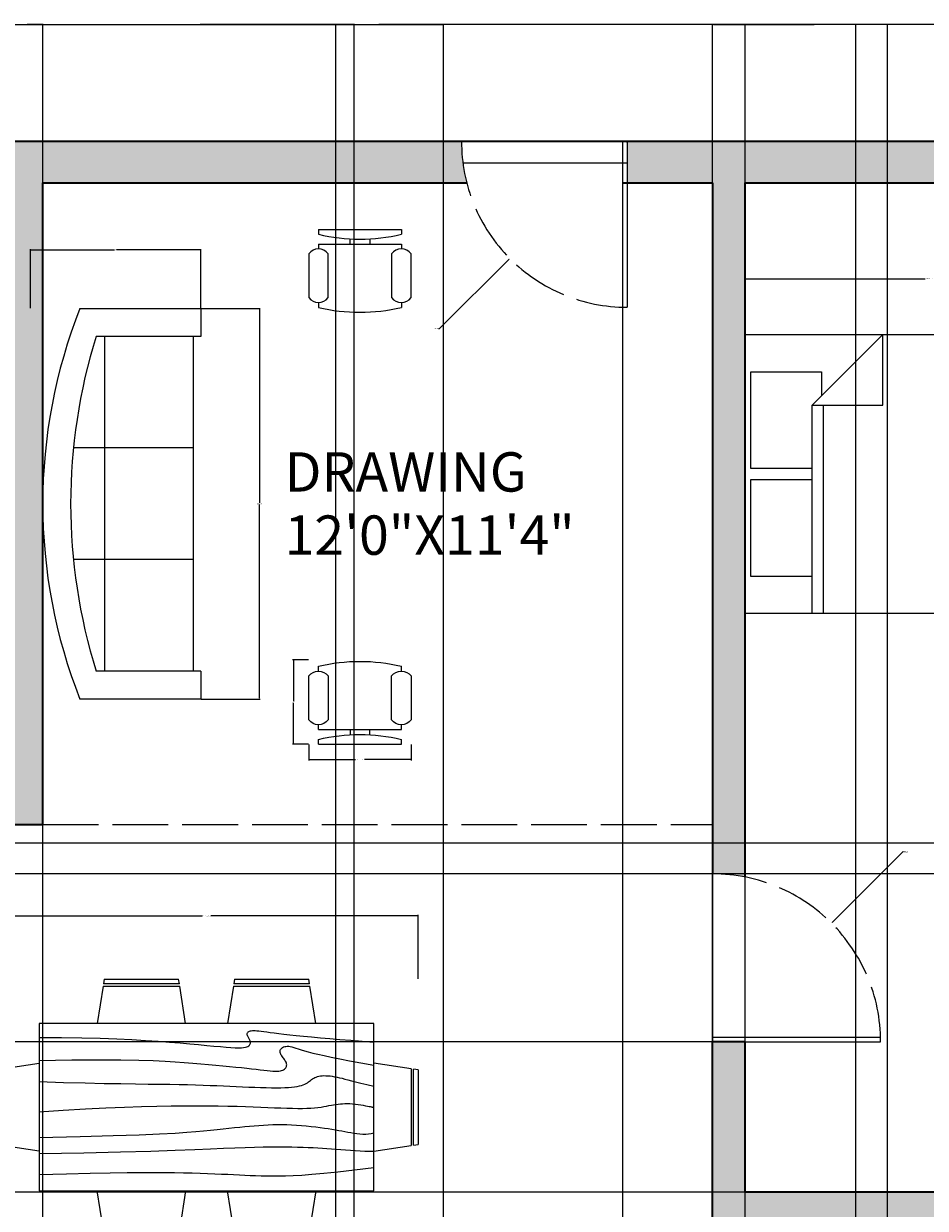
# Model space of a CAD drawing. Units: inches. Extents: x -12 to 539, y -477 to 51.
# Tile 5 of 6: x 173 to 367, y -203 to 51. Entities that reach past the tile are written whole.
import ezdxf

# ---------------------------------------------------------------- set-up
doc = ezdxf.new("R2010")
doc.units = ezdxf.units.IN
doc.header["$MEASUREMENT"] = 0
doc.linetypes.add('ACAD_ISO02W100', pattern=[15, 12, -3])
for name, color, linetype, lineweight in [('A-ANNO-DIMS', 2, 'Continuous', 18), ('A-AREA-IDEN', 7, 'Continuous', 18), ('A-DOOR', 4, 'Continuous', 25), ('A-DOOR-SWNG', 4, 'ACAD_ISO02W100', 13), ('A-FURN', 8, 'Continuous', 18), ('A-WALL', 7, 'Continuous', 35), ('A-WALL-OVHD', 7, 'ACAD_ISO02W100', 18)]:
    doc.layers.add(name, color=color, linetype=linetype, lineweight=lineweight)
doc.layers.add('A-WALL-PATT', color=252, linetype='Continuous', lineweight=13, true_color=0x939598)
doc.styles.get("Standard").update_dxf_attribs({"font": 'arial.ttf'})
doc.dimstyles.get("Standard").update_dxf_attribs({"dimtxt": 0.18, "dimasz": 0.18, "dimexe": 0.18, "dimexo": 0.0625, "dimgap": 0.09, "dimtad": 0, "dimtih": 1, "dimtoh": 1, "dimdec": 0, "dimzin": 0, "dimdsep": 46, "dimlunit": 3, "dimtxsty": 'Standard', "dimcen": 0.09, "dimadec": 0, "dimazin": 0, "dimtfac": 1, "dimtdec": 0, "dimtofl": 0, "dimtmove": 0, "dimatfit": 3, "dimfxl": 1, "dimtolj": 1, "dimtzin": 0, "dimarcsym": 0})

# ---------------------------------------------------------------- blocks, each defined once
blk = doc.blocks.new('Sofa - Roundback 7 ft.')
for p, q in [((-12.00002, -32.4421), (-12.00003, -6.5971)), ((11.99997, -32.4421), (11.99998, -6.5971)), ((-36.000027, -34), (-36.000027, -11.4696)), ((35.99998, -34), (35.99998, -11.4696)), ((-35.999844, -13.3819), (35.9998, -13.3819)), ((-36.000027, -32.4421), (35.99998, -32.4421))]:
    blk.add_line(p, q)
for points in [[(-36.000027, -34), (-42.000027, -34), (-42.000027, -8)], [(41.99998, -8), (41.99998, -34), (35.99998, -34)]]:
    blk.add_lwpolyline(points)
for centre, radius, start, end in [((0, -114.25), 114.25, 68.43141, 111.5686), ((-0.00001, -127.1968), 121.1968, 72.72033, 107.2797)]:
    blk.add_arc(centre, radius, start, end)
blk = doc.blocks.new('Chair - Desk')
for p, q in [((-8.5, 0), (-8.5, -1)), ((-8.5, 0), (8.5, 0)), ((8.5, 0), (8.5, -1)), ((-2, -3), (-2, -1.9355)), ((2, -1.9576), (2, -3)), ((-8.5, -3), (-8.5, -4)), ((-8.5, -3), (8.5, -3)), ((8.5, -3), (8.5, -4)), ((-10.5, -5), (-10.5, -14)), ((-6.5, -14), (-6.5, -5)), ((6.5, -5), (6.5, -14)), ((10.5, -14), (10.5, -5)), ((-8.5, -15), (-8.5, -16)), ((8.5, -15), (8.5, -16))]:
    blk.add_line(p, q)
for centre, radius, start, end in [((0, 34.625), 36.625, 256.5803, 283.4197), ((-8.5, -6.5), 2.5, 36.8699, 143.1301), ((8.5, -6.5), 2.5, 36.8699, 143.1301), ((-8.5, -12.5), 2.5, 216.8699, 323.1301), ((8.5, -12.5), 2.5, 216.8699, 323.1301), ((0, 19.625), 36.625, 256.5803, 283.4197)]:
    blk.add_arc(centre, radius, start, end)
blk = doc.blocks.new('Bed - Queen')
for p, q in [((0, -80.00003), (0, 0)), ((0, 0), (59.99999, 0)), ((59.99999, 0), (59.99999, -80.00003)), ((7.99999, -1.2), (28.79998, -1.2)), ((7.99999, -14.4), (7.99999, -1.2)), ((28.79998, -1.2), (28.79998, -14.4)), ((31.19999, -1.2), (51.99999, -1.2)), ((31.19999, -14.4), (31.19999, -1.2)), ((51.99999, -1.2), (51.99999, -16.4)), ((0, -14.4), (44.8, -14.4)), ((59.99999, -29.6), (44.8, -14.4)), ((44.8, -14.4), (44.8, -29.6)), ((44.8, -16.8), (0, -16.8)), ((51.99999, -16.4), (46.79936, -16.4)), ((44.8, -29.6), (59.99999, -29.6)), ((59.99999, -80.00003), (0, -80.00003))]:
    blk.add_line(p, q)
blk = doc.blocks.new('Dining Set - 36 x 72 in.')
for p, q in [((-22.2343, 26.00059), (-23.4847, 17.99762)), ((-22.2304, 26), (-5.7608, 26)), ((-22, 27.5), (-22.1562, 26.50042)), ((-5.8416, 26.5), (-22.1534, 26.5)), ((-22, 27.5), (-6, 27.5)), ((-5.8437, 26.49966), (-6, 27.5)), ((-4.5152, 17.99762), (-5.7655, 25.99926)), ((5.7657, 26.00059), (4.5153, 17.99762)), ((5.7696, 26), (22.2392, 26)), ((6, 27.5), (5.8438, 26.50042)), ((22.1584, 26.5), (5.8466, 26.5)), ((6, 27.5), (22, 27.5)), ((22.1563, 26.49966), (22, 27.5)), ((23.4848, 17.99762), (22.2345, 25.99926)), ((36, 18), (-36, 18)), ((-36, 18), (-36, -18)), ((36, -18), (36, 18)), ((-45.5, 8), (-44.5004, 8.15617)), ((-45.5, 8), (-45.5, -8)), ((-44.5, -8.15843), (-44.5, 8.15338)), ((-44.0006, 8.23428), (-35.9976, 9.48474)), ((-44, 8.23041), (-44, -8.23915)), ((44.0006, 8.23428), (35.9976, 9.48474)), ((44, 8.23041), (44, -8.23915)), ((44.5, -8.15843), (44.5, 8.15338)), ((45.5, 8), (44.5005, 8.15617)), ((45.5, 8), (45.5, -8)), ((-44.4997, -8.15631), (-45.5, -8)), ((-35.9976, -9.48476), (-43.9993, -8.2345)), ((35.9976, -9.48476), (43.9993, -8.2345)), ((44.4997, -8.15631), (45.5, -8)), ((-36, -18), (36, -18)), ((-22.2343, -26.0006), (-23.4847, -17.99762)), ((-4.5152, -17.99762), (-5.7655, -25.99928)), ((5.7657, -26.0006), (4.5153, -17.99762)), ((23.4848, -17.99762), (22.2345, -25.99928)), ((-22.2304, -26), (-5.7608, -26)), ((-22, -27.5), (-22.1562, -26.50044)), ((-5.8416, -26.5), (-22.1534, -26.5)), ((-22, -27.5), (-6, -27.5)), ((-5.8437, -26.49967), (-6, -27.5)), ((5.7696, -26), (22.2392, -26)), ((6, -27.5), (5.8438, -26.50044)), ((22.1584, -26.5), (5.8466, -26.5)), ((6, -27.5), (22, -27.5)), ((22.1563, -26.49967), (22, -27.5))]:
    blk.add_line(p, q)
for points in [[(-36, 15), (-31.1772, 14.97754), (-26.8079, 14.91406), (-22.8538, 14.81543), (-19.276, 14.6875), (-16.0362, 14.53613), (-13.0957, 14.36718), (-10.4159, 14.18652), (-7.9583, 14), (-5.6904, 13.81315), (-3.6035, 13.63021), (-1.6954, 13.45508), (0.0365, 13.29166), (1.5945, 13.14388), (2.9811, 13.01562), (4.1988, 12.9108), (5.25, 12.83333), (6.1393, 12.78613), (6.8802, 12.76823), (7.4883, 12.77767), (7.9792, 12.8125), (8.3685, 12.87077), (8.6719, 12.95052), (8.9049, 13.0498), (9.0833, 13.16666), (9.2205, 13.29899), (9.3216, 13.44401), (9.3895, 13.59879), (9.4271, 13.76041), (9.4373, 13.92594), (9.4232, 14.09245), (9.3875, 14.257), (9.3333, 14.41666), (9.2638, 14.56917), (9.1836, 14.71484), (9.0975, 14.85465), (9.0104, 14.98958), (8.9272, 15.1206), (8.8529, 15.2487), (8.7922, 15.37483), (8.75, 15.5), (8.7305, 15.62467), (8.7344, 15.74739), (8.7617, 15.86621), (8.8125, 15.97916), (8.8867, 16.08431), (8.9844, 16.17968), (9.1055, 16.26334), (9.25, 16.33333), (9.4189, 16.38802), (9.6172, 16.42708), (9.8506, 16.45052), (10.125, 16.45833), (10.4463, 16.45052), (10.8203, 16.42708), (11.2529, 16.38802), (11.75, 16.33333), (12.3184, 16.26318), (12.9694, 16.17838), (13.7151, 16.07991), (14.5677, 15.96875), (15.5395, 15.84586), (16.6426, 15.71224), (17.8893, 15.56884), (19.2917, 15.41666), (20.859, 15.25667), (22.5879, 15.08984), (24.4721, 14.91715), (26.5052, 14.73958), (28.6809, 14.5581), (30.9929, 14.3737), (33.4347, 14.18733), (36, 14)], [(-36, 10), (-28.9766, 10.14274), (-23.1725, 10.20442), (-18.4241, 10.19775), (-14.5677, 10.13541), (-11.4399, 10.03011), (-8.877, 9.89453), (-6.7154, 9.74137), (-4.7917, 9.58333), (-2.9698, 9.43082), (-1.2246, 9.28515), (0.4415, 9.14534), (2.026, 9.01041), (3.5266, 8.87939), (4.9408, 8.7513), (6.266, 8.62516), (7.5, 8.5), (8.6411, 8.37549), (9.6914, 8.2539), (10.6538, 8.13818), (11.5312, 8.03125), (12.3267, 7.93603), (13.043, 7.85547), (13.6831, 7.79248), (14.25, 7.75), (14.7471, 7.7303), (15.1797, 7.73307), (15.5537, 7.75732), (15.875, 7.80208), (16.1494, 7.86637), (16.3828, 7.94922), (16.5811, 8.04964), (16.75, 8.16666), (16.8944, 8.29915), (17.0143, 8.44531), (17.1089, 8.60319), (17.1771, 8.77083), (17.218, 8.94629), (17.2305, 9.1276), (17.2137, 9.31282), (17.1667, 9.5), (17.0895, 9.6875), (16.987, 9.875), (16.8649, 10.0625), (16.7292, 10.25), (16.5856, 10.4375), (16.4401, 10.625), (16.2985, 10.8125), (16.1667, 11), (16.05, 11.18733), (15.9518, 11.3737), (15.8752, 11.5581), (15.8229, 11.73958), (15.798, 11.91715), (15.8034, 12.08984), (15.842, 12.25667), (15.9167, 12.41666), (16.0295, 12.56836), (16.1784, 12.70833), (16.3605, 12.83268), (16.5729, 12.9375), (16.8127, 13.01888), (17.0768, 13.07291), (17.3625, 13.0957), (17.6667, 13.08333), (17.9894, 13.03312), (18.3418, 12.94726), (18.7382, 12.82918), (19.1927, 12.68229), (19.7195, 12.51001), (20.3327, 12.31575), (21.0465, 12.10294), (21.875, 11.875), (22.8357, 11.63354), (23.959, 11.37304), (25.2786, 11.08618), (26.8282, 10.76562), (28.6414, 10.40405), (30.752, 9.99414), (33.1936, 9.52856), (36, 9)], [(-36, 5.5), (-30.7157, 5.3348), (-26.069, 5.20963), (-21.9946, 5.11767), (-18.4271, 5.05208), (-15.3009, 5.00602), (-12.5508, 4.97265), (-10.1112, 4.94515), (-7.9167, 4.91666), (-5.909, 4.88167), (-4.0586, 4.83984), (-2.3429, 4.79215), (-0.7396, 4.73958), (0.7739, 4.6831), (2.22, 4.6237), (3.6213, 4.56233), (5, 4.5), (6.373, 4.43782), (7.7344, 4.3776), (9.0723, 4.32129), (10.375, 4.27083), (11.6309, 4.22819), (12.8281, 4.19531), (13.9551, 4.17415), (15, 4.16666), (15.954, 4.17448), (16.819, 4.19791), (17.6001, 4.23698), (18.3021, 4.29166), (18.9299, 4.36198), (19.4883, 4.44791), (19.9823, 4.54948), (20.4167, 4.66666), (20.7969, 4.79899), (21.1302, 4.94401), (21.4245, 5.09879), (21.6875, 5.26041), (21.9271, 5.42594), (22.1511, 5.59245), (22.3672, 5.757), (22.5834, 5.91666), (22.8065, 6.06868), (23.0404, 6.21093), (23.2879, 6.34147), (23.5521, 6.45833), (23.8358, 6.55957), (24.142, 6.64323), (24.4735, 6.70735), (24.8334, 6.75), (25.2235, 6.76969), (25.642, 6.76692), (26.0858, 6.74267), (26.5521, 6.69791), (27.0379, 6.63362), (27.5404, 6.55078), (28.0565, 6.45036), (28.5834, 6.33333), (29.1242, 6.19987), (29.7071, 6.04687), (30.3661, 5.87044), (31.1354, 5.66666), (32.0493, 5.43164), (33.142, 5.16146), (34.4475, 4.85221), (36, 4.5)], [(-36, -1), (-30.7915, -0.6591), (-26.0195, -0.38216), (-21.6519, -0.16284), (-17.6563, 0.00521), (-14.0005, 0.12833), (-10.6523, 0.21289), (-7.5796, 0.26522), (-4.75, 0.29166), (-2.134, 0.29793), (0.2878, 0.28711), (2.5317, 0.26163), (4.6146, 0.22396), (6.5529, 0.17651), (8.3633, 0.12174), (10.0623, 0.06209), (11.6667, 0), (13.1899, -0.06201), (14.6341, -0.1211), (15.9982, -0.17432), (17.2813, -0.21875), (18.4823, -0.25147), (19.6003, -0.26953), (20.6343, -0.27002), (21.5834, -0.25), (22.4481, -0.20768), (23.2357, -0.14584), (23.9549, -0.06836), (24.6146, 0.02083), (25.2235, 0.11784), (25.7904, 0.21875), (26.3241, 0.31966), (26.8334, 0.41666), (27.3265, 0.50618), (27.8099, 0.58593), (28.2894, 0.65397), (28.7709, 0.70833), (29.2601, 0.74707), (29.763, 0.76823), (30.2855, 0.76985), (30.8334, 0.75), (31.4088, 0.70784), (31.9994, 0.64713), (32.589, 0.57275), (33.1615, 0.48958), (33.7008, 0.4025), (34.1908, 0.3164), (34.6153, 0.23616), (34.9584, 0.16666), (35.2099, 0.11165), (35.3848, 0.07031), (35.504, 0.04069), (35.5886, 0.02083), (35.6594, 0.00879), (35.7377, 0.0026), (35.8442, 0.00032), (36, 0)], [(-36, -6.5), (-27.1843, -6.31267), (-20.084, -6.1263), (-14.469, -5.9419), (-10.1094, -5.76042), (-6.7752, -5.58285), (-4.2363, -5.41016), (-2.2629, -5.24333), (-0.625, -5.08334), (0.8708, -4.93099), (2.2715, -4.78646), (3.5872, -4.64974), (4.8281, -4.52084), (6.0046, -4.39974), (7.127, -4.28646), (8.2053, -4.18099), (9.25, -4.08334), (10.2705, -3.99382), (11.2734, -3.91407), (12.2647, -3.84603), (13.25, -3.79167), (14.2354, -3.75293), (15.2266, -3.73177), (16.2295, -3.73015), (17.25, -3.75), (18.2912, -3.79248), (19.3451, -3.85547), (20.4009, -3.93604), (21.4479, -4.03125), (22.4754, -4.13819), (23.4727, -4.25391), (24.4289, -4.37549), (25.3334, -4.5), (26.1785, -4.62492), (26.9694, -4.74935), (27.7145, -4.87281), (28.4219, -4.99479), (29.1, -5.11483), (29.7572, -5.23242), (30.4016, -5.34709), (31.0417, -5.45834), (31.6837, -5.56437), (32.3262, -5.65821), (32.9658, -5.73153), (33.599, -5.77604), (34.2224, -5.78345), (34.8327, -5.74545), (35.4264, -5.65373), (36, -5.5)], [(-36, -10), (-26.4022, -9.81299), (-18.4675, -9.62891), (-11.9839, -9.45069), (-6.7396, -9.28125), (-2.5226, -9.12354), (0.8789, -8.98047), (3.6769, -8.85498), (6.0833, -8.75), (8.2767, -8.66765), (10.3021, -8.60677), (12.1712, -8.56543), (13.8958, -8.54167), (15.4876, -8.53353), (16.9583, -8.53907), (18.3197, -8.55632), (19.5834, -8.58334), (20.7616, -8.61841), (21.8685, -8.66081), (22.9188, -8.71004), (23.9271, -8.76563), (24.9081, -8.82707), (25.8763, -8.89388), (26.8465, -8.96558), (27.8334, -9.04167), (28.8474, -9.12118), (29.8828, -9.20117), (30.93, -9.27824), (31.9792, -9.34896), (33.0205, -9.40991), (34.0443, -9.45768), (35.0407, -9.48885), (36, -9.5)], [(-36, -14.5), (-30.0881, -14.33513), (-25.0332, -14.21224), (-20.7312, -14.12647), (-17.0781, -14.07292), (-13.97, -14.04671), (-11.3027, -14.04297), (-8.9724, -14.05681), (-6.875, -14.08334), (-4.9224, -14.11833), (-3.0905, -14.16016), (-1.3709, -14.20785), (0.2448, -14.26042), (1.7647, -14.3169), (3.1973, -14.3763), (4.5507, -14.43767), (5.8333, -14.5), (7.0554, -14.5621), (8.235, -14.62175), (9.3922, -14.67652), (10.5469, -14.72396), (11.7192, -14.76164), (12.929, -14.78711), (14.1965, -14.79794), (15.5417, -14.79167), (16.9933, -14.76424), (18.6152, -14.70508), (20.4804, -14.60197), (22.6615, -14.44271), (25.2312, -14.21509), (28.2624, -13.9069), (31.8277, -13.50594), (36, -13)]]:
    blk.add_lwpolyline(points)
blk = doc.blocks.new('*D9')
at = {"layer": 'A-ANNO-DIMS', "color": 0, "lineweight": -2, "transparency": 16777216}
for p, q in [((328.1, -15.53), (328.1, -3.41)), ((328.28, -3.59), (366.8, -3.59)), ((407.92, -3.59), (369.41, -3.59)), ((408.1, -15.53), (408.1, -3.41))]:
    blk.add_line(p, q, dxfattribs=at)
at = {"layer": 'A-ANNO-DIMS', "color": 0, "transparency": 16777216}
for points in [[(328.28, -3.56), (328.28, -3.62), (328.1, -3.59)], [(407.92, -3.56), (407.92, -3.62), (408.1, -3.59)]]:
    blk.add_solid(points, dxfattribs=at)
at = {"layer": 'Defpoints', "color": 0, "transparency": 16777216}
for p in [(328.1, -3.59), (328.1, -15.59), (408.1, -15.59)]:
    blk.add_point(p, dxfattribs=at)
at = {"layer": 'A-ANNO-DIMS', "color": 0, "transparency": 16777216, "insert": (368.1, -3.59), "char_height": 0.18, "attachment_point": 5}
blk.add_mtext('\\A1;QUEEN BED 80 TYP.', dxfattribs=at)
blk = doc.blocks.new('*D11')
at = {"layer": 'A-ANNO-DIMS', "color": 0, "lineweight": -2, "transparency": 16777216}
for p, q in [((234.28, -103.76), (234.28, -107.18)), ((256.31, -103.76), (256.31, -107.18)), ((234.46, -107), (244.34, -107)), ((256.13, -107), (246.25, -107))]:
    blk.add_line(p, q, dxfattribs=at)
at = {"layer": 'A-ANNO-DIMS', "color": 0, "transparency": 16777216}
for points in [[(234.46, -106.97), (234.46, -107.03), (234.28, -107)], [(256.13, -106.97), (256.13, -107.03), (256.31, -107)]]:
    blk.add_solid(points, dxfattribs=at)
at = {"layer": 'Defpoints', "color": 0, "transparency": 16777216}
for p in [(234.28, -103.7), (256.31, -103.7), (256.31, -107)]:
    blk.add_point(p, dxfattribs=at)
at = {"layer": 'A-ANNO-DIMS', "color": 0, "transparency": 16777216, "insert": (245.3, -107), "char_height": 0.18, "attachment_point": 5}
blk.add_mtext('\\A1;CHAIR 22 TYP.', dxfattribs=at)
blk = doc.blocks.new('*D12')
at = {"layer": 'A-ANNO-DIMS', "color": 0, "lineweight": -2, "transparency": 16777216}
for p, q in [((234.22, -85.52), (230.8, -85.52)), ((230.98, -85.7), (230.98, -94.43)), ((230.98, -103.52), (230.98, -94.79)), ((234.22, -103.7), (230.8, -103.7))]:
    blk.add_line(p, q, dxfattribs=at)
at = {"layer": 'A-ANNO-DIMS', "color": 0, "transparency": 16777216}
for points in [[(230.95, -85.7), (231.01, -85.7), (230.98, -85.52)], [(230.95, -103.52), (231.01, -103.52), (230.98, -103.7)]]:
    blk.add_solid(points, dxfattribs=at)
at = {"layer": 'Defpoints', "color": 0, "transparency": 16777216}
for p in [(234.28, -85.52), (230.98, -103.7), (234.28, -103.7)]:
    blk.add_point(p, dxfattribs=at)
at = {"layer": 'A-ANNO-DIMS', "color": 0, "transparency": 16777216, "insert": (230.98, -94.61), "char_height": 0.18, "attachment_point": 5}
blk.add_mtext('\\A1;18 TYP.', dxfattribs=at)
blk = doc.blocks.new('*D29')
at = {"layer": 'A-ANNO-DIMS', "color": 0, "lineweight": -2, "transparency": 16777216}
for p, q in [((166.81, -154.17), (166.81, -140.4)), ((166.99, -140.58), (211.36, -140.58)), ((257.63, -140.58), (213.27, -140.58)), ((257.81, -154.17), (257.81, -140.4))]:
    blk.add_line(p, q, dxfattribs=at)
at = {"layer": 'A-ANNO-DIMS', "color": 0, "transparency": 16777216}
for points in [[(166.99, -140.55), (166.99, -140.61), (166.81, -140.58)], [(257.63, -140.55), (257.63, -140.61), (257.81, -140.58)]]:
    blk.add_solid(points, dxfattribs=at)
at = {"layer": 'Defpoints', "color": 0, "transparency": 16777216}
for p in [(257.81, -140.58), (166.81, -154.23), (257.81, -154.23)]:
    blk.add_point(p, dxfattribs=at)
at = {"layer": 'A-ANNO-DIMS', "color": 0, "transparency": 16777216, "insert": (212.31, -140.58), "char_height": 0.18, "attachment_point": 5}
blk.add_mtext('\\A1;DINING SET 91', dxfattribs=at)
blk = doc.blocks.new('*D31')
at = {"layer": 'A-ANNO-DIMS', "color": 0, "lineweight": -2, "transparency": 16777216}
for p, q in [((211.17, -9.99), (223.88, -9.99)), ((223.7, -10.17), (223.7, -51.8)), ((223.7, -93.81), (223.7, -52.17)), ((211.17, -93.99), (223.88, -93.99))]:
    blk.add_line(p, q, dxfattribs=at)
at = {"layer": 'A-ANNO-DIMS', "color": 0, "transparency": 16777216}
for points in [[(223.67, -10.17), (223.73, -10.17), (223.7, -9.99)], [(223.67, -93.81), (223.73, -93.81), (223.7, -93.99)]]:
    blk.add_solid(points, dxfattribs=at)
at = {"layer": 'Defpoints', "color": 0, "transparency": 16777216}
for p in [(211.1, -9.99), (223.7, -9.99), (211.1, -93.99)]:
    blk.add_point(p, dxfattribs=at)
at = {"layer": 'A-ANNO-DIMS', "color": 0, "transparency": 16777216, "insert": (223.7, -51.99), "char_height": 0.18, "attachment_point": 5}
blk.add_mtext('\\A1;SOFA 84', dxfattribs=at)
blk = doc.blocks.new('*D32')
at = {"layer": 'A-ANNO-DIMS', "color": 0, "lineweight": -2, "transparency": 16777216}
for p, q in [((174.44, -9.93), (174.44, 2.79)), ((174.62, 2.61), (192.55, 2.61)), ((210.92, 2.61), (192.99, 2.61)), ((211.1, -9.93), (211.1, 2.79))]:
    blk.add_line(p, q, dxfattribs=at)
at = {"layer": 'A-ANNO-DIMS', "color": 0, "transparency": 16777216}
for points in [[(174.62, 2.64), (174.62, 2.58), (174.44, 2.61)], [(210.92, 2.64), (210.92, 2.58), (211.1, 2.61)]]:
    blk.add_solid(points, dxfattribs=at)
at = {"layer": 'Defpoints', "color": 0, "transparency": 16777216}
for p in [(174.44, 2.61), (174.44, -9.99), (211.1, -9.99)]:
    blk.add_point(p, dxfattribs=at)
at = {"layer": 'A-ANNO-DIMS', "color": 0, "transparency": 16777216, "insert": (192.77, 2.61), "char_height": 0.18, "attachment_point": 5}
blk.add_mtext('\\A1;37', dxfattribs=at)
blk = doc.blocks.new('*D35')
at = {"layer": 'A-ANNO-DIMS', "color": 0, "lineweight": -2, "transparency": 16777216}
for p, q in [((301.71, 16.95), (301.71, -477.23)), ((321.1, 16.95), (321.1, -477.23)), ((301.89, -477.05), (311.02, -477.05)), ((320.92, -477.05), (311.79, -477.05))]:
    blk.add_line(p, q, dxfattribs=at)
at = {"layer": 'A-ANNO-DIMS', "color": 0, "transparency": 16777216}
for points in [[(301.89, -477.02), (301.89, -477.08), (301.71, -477.05)], [(320.92, -477.02), (320.92, -477.08), (321.1, -477.05)]]:
    blk.add_solid(points, dxfattribs=at)
at = {"layer": 'Defpoints', "color": 0, "transparency": 16777216}
for p in [(301.71, 17.01), (321.1, 17.01), (321.1, -477.05)]:
    blk.add_point(p, dxfattribs=at)
at = {"layer": 'A-ANNO-DIMS', "color": 0, "transparency": 16777216, "insert": (311.41, -477.05), "char_height": 0.18, "attachment_point": 5}
blk.add_mtext('\\A1;19.39', dxfattribs=at)
blk = doc.blocks.new('*D37')
at = {"layer": 'A-ANNO-DIMS', "color": 0, "lineweight": -2, "transparency": 16777216}
for p, q in [((13.1, 26.07), (13.1, 51.25)), ((13.28, 51.07), (263.15, 51.07)), ((513.81, 51.07), (263.94, 51.07)), ((513.99, -124.93), (513.99, 51.25))]:
    blk.add_line(p, q, dxfattribs=at)
at = {"layer": 'A-ANNO-DIMS', "color": 0, "transparency": 16777216}
for points in [[(13.28, 51.1), (13.28, 51.04), (13.1, 51.07)], [(513.81, 51.1), (513.81, 51.04), (513.99, 51.07)]]:
    blk.add_solid(points, dxfattribs=at)
at = {"layer": 'Defpoints', "color": 0, "transparency": 16777216}
for p in [(513.99, 51.07), (13.1, 26.01), (513.99, -124.99)]:
    blk.add_point(p, dxfattribs=at)
at = {"layer": 'A-ANNO-DIMS', "color": 0, "transparency": 16777216, "insert": (263.54, 51.07), "char_height": 0.18, "attachment_point": 5}
blk.add_mtext('\\A1;500.9', dxfattribs=at)
blk = doc.blocks.new('*D42')
at = {"layer": 'A-ANNO-DIMS', "color": 0, "lineweight": -2, "transparency": 16777216}
for p, q in [((177.1, -442.93), (177.1, 51.25)), ((177.28, 51.07), (248.82, 51.07)), ((320.92, 51.07), (249.38, 51.07)), ((321.1, -442.93), (321.1, 51.25))]:
    blk.add_line(p, q, dxfattribs=at)
at = {"layer": 'A-ANNO-DIMS', "color": 0, "transparency": 16777216}
for points in [[(177.28, 51.1), (177.28, 51.04), (177.1, 51.07)], [(320.92, 51.1), (320.92, 51.04), (321.1, 51.07)]]:
    blk.add_solid(points, dxfattribs=at)
at = {"layer": 'Defpoints', "color": 0, "transparency": 16777216}
for p in [(321.1, 51.07), (177.1, -442.99), (321.1, -442.99)]:
    blk.add_point(p, dxfattribs=at)
at = {"layer": 'A-ANNO-DIMS', "color": 0, "transparency": 16777216, "insert": (249.1, 51.07), "char_height": 0.18, "attachment_point": 5}
blk.add_mtext('\\A1;144', dxfattribs=at)
blk = doc.blocks.new('*D46')
at = {"layer": 'A-ANNO-DIMS', "color": 0, "lineweight": -2, "transparency": 16777216}
for p, q in [((170.1, 17.07), (170.1, 51.25)), ((170.28, 51.07), (173.45, 51.07)), ((176.92, 51.07), (173.75, 51.07)), ((177.1, 17.07), (177.1, 51.25))]:
    blk.add_line(p, q, dxfattribs=at)
at = {"layer": 'A-ANNO-DIMS', "color": 0, "transparency": 16777216}
for points in [[(170.28, 51.1), (170.28, 51.04), (170.1, 51.07)], [(176.92, 51.1), (176.92, 51.04), (177.1, 51.07)]]:
    blk.add_solid(points, dxfattribs=at)
at = {"layer": 'Defpoints', "color": 0, "transparency": 16777216}
for p in [(177.1, 51.07), (170.1, 17.01), (177.1, 17.01)]:
    blk.add_point(p, dxfattribs=at)
at = {"layer": 'A-ANNO-DIMS', "color": 0, "transparency": 16777216, "insert": (173.6, 51.07), "char_height": 0.18, "attachment_point": 5}
blk.add_mtext('\\A1;7', dxfattribs=at)
blk = doc.blocks.new('*D50')
at = {"layer": 'A-ANNO-DIMS', "color": 0, "lineweight": -2, "transparency": 16777216}
for p, q in [((321.04, -167.71), (-12.14, -167.71)), ((-11.96, -167.89), (-11.96, -183.67)), ((-11.96, -199.81), (-11.96, -184.03)), ((328.04, -199.99), (-12.14, -199.99))]:
    blk.add_line(p, q, dxfattribs=at)
at = {"layer": 'A-ANNO-DIMS', "color": 0, "transparency": 16777216}
for points in [[(-11.99, -167.89), (-11.93, -167.89), (-11.96, -167.71)], [(-11.99, -199.81), (-11.93, -199.81), (-11.96, -199.99)]]:
    blk.add_solid(points, dxfattribs=at)
at = {"layer": 'Defpoints', "color": 0, "transparency": 16777216}
for p in [(-11.96, -167.71), (321.1, -167.71), (328.1, -199.99)]:
    blk.add_point(p, dxfattribs=at)
at = {"layer": 'A-ANNO-DIMS', "color": 0, "transparency": 16777216, "insert": (-11.96, -183.85), "char_height": 0.18, "attachment_point": 5}
blk.add_mtext('\\A1;32.274', dxfattribs=at)
blk = doc.blocks.new('*D51')
at = {"layer": 'A-ANNO-DIMS', "color": 0, "lineweight": -2, "transparency": 16777216}
for p, q in [((328.1, -323.93), (328.1, 51.25)), ((328.28, 51.07), (342.93, 51.07)), ((358.5, 51.07), (343.85, 51.07)), ((358.68, -323.93), (358.68, 51.25))]:
    blk.add_line(p, q, dxfattribs=at)
at = {"layer": 'A-ANNO-DIMS', "color": 0, "transparency": 16777216}
for points in [[(328.28, 51.1), (328.28, 51.04), (328.1, 51.07)], [(358.5, 51.1), (358.5, 51.04), (358.68, 51.07)]]:
    blk.add_solid(points, dxfattribs=at)
at = {"layer": 'Defpoints', "color": 0, "transparency": 16777216}
for p in [(358.68, 51.07), (328.1, -323.99), (358.68, -323.99)]:
    blk.add_point(p, dxfattribs=at)
at = {"layer": 'A-ANNO-DIMS', "color": 0, "transparency": 16777216, "insert": (343.39, 51.07), "char_height": 0.18, "attachment_point": 5}
blk.add_mtext('\\A1;30.574', dxfattribs=at)
blk = doc.blocks.new('*D53')
at = {"layer": 'A-ANNO-DIMS', "color": 0, "lineweight": -2, "transparency": 16777216}
for p, q in [((379.04, -124.99), (-12.14, -124.99)), ((-11.96, -125.17), (-11.96, -128.09)), ((-11.96, -131.38), (-11.96, -128.46)), ((379.04, -131.56), (-12.14, -131.56))]:
    blk.add_line(p, q, dxfattribs=at)
at = {"layer": 'A-ANNO-DIMS', "color": 0, "transparency": 16777216}
for points in [[(-11.99, -125.17), (-11.93, -125.17), (-11.96, -124.99)], [(-11.99, -131.38), (-11.93, -131.38), (-11.96, -131.56)]]:
    blk.add_solid(points, dxfattribs=at)
at = {"layer": 'Defpoints', "color": 0, "transparency": 16777216}
for p in [(379.1, -124.99), (-11.96, -131.56), (379.1, -131.56)]:
    blk.add_point(p, dxfattribs=at)
at = {"layer": 'A-ANNO-DIMS', "color": 0, "transparency": 16777216, "insert": (-11.96, -128.27), "char_height": 0.18, "attachment_point": 5}
blk.add_mtext('\\A1;6.575', dxfattribs=at)
blk = doc.blocks.new('*D56')
at = {"layer": 'A-ANNO-DIMS', "color": 0, "lineweight": -2, "transparency": 16777216}
for p, q in [((321.1, -256.48), (321.1, 51.25)), ((321.28, 51.07), (336.1, 51.07)), ((351.7, 51.07), (336.89, 51.07)), ((351.88, -256.48), (351.88, 51.25))]:
    blk.add_line(p, q, dxfattribs=at)
at = {"layer": 'A-ANNO-DIMS', "color": 0, "transparency": 16777216}
for points in [[(321.28, 51.1), (321.28, 51.04), (321.1, 51.07)], [(351.7, 51.1), (351.7, 51.04), (351.88, 51.07)]]:
    blk.add_solid(points, dxfattribs=at)
at = {"layer": 'Defpoints', "color": 0, "transparency": 16777216}
for p in [(351.88, 51.07), (321.1, -256.55), (351.88, -256.55)]:
    blk.add_point(p, dxfattribs=at)
at = {"layer": 'A-ANNO-DIMS', "color": 0, "transparency": 16777216, "insert": (336.49, 51.07), "char_height": 0.18, "attachment_point": 5}
blk.add_mtext('\\A1;30.78', dxfattribs=at)
blk = doc.blocks.new('*D58')
at = {"layer": 'A-ANNO-DIMS', "color": 0, "lineweight": -2, "transparency": 16777216}
for p, q in [((177.1, -250.93), (177.1, 51.25)), ((177.28, 51.07), (210.17, 51.07)), ((243.85, 51.07), (210.96, 51.07)), ((244.03, -250.93), (244.03, 51.25))]:
    blk.add_line(p, q, dxfattribs=at)
at = {"layer": 'A-ANNO-DIMS', "color": 0, "transparency": 16777216}
for points in [[(177.28, 51.1), (177.28, 51.04), (177.1, 51.07)], [(243.85, 51.1), (243.85, 51.04), (244.03, 51.07)]]:
    blk.add_solid(points, dxfattribs=at)
at = {"layer": 'Defpoints', "color": 0, "transparency": 16777216}
for p in [(244.03, 51.07), (177.1, -250.99), (244.03, -250.99)]:
    blk.add_point(p, dxfattribs=at)
at = {"layer": 'A-ANNO-DIMS', "color": 0, "transparency": 16777216, "insert": (210.56, 51.07), "char_height": 0.18, "attachment_point": 5}
blk.add_mtext('\\A1;66.92', dxfattribs=at)
blk = doc.blocks.new('*D59')
at = {"layer": 'A-ANNO-DIMS', "color": 0, "lineweight": -2, "transparency": 16777216}
for p, q in [((240.14, -279.15), (240.14, 51.25)), ((240.32, 51.07), (251.3, 51.07)), ((263.07, 51.07), (252.09, 51.07)), ((263.25, -279.15), (263.25, 51.25))]:
    blk.add_line(p, q, dxfattribs=at)
at = {"layer": 'A-ANNO-DIMS', "color": 0, "transparency": 16777216}
for points in [[(240.32, 51.1), (240.32, 51.04), (240.14, 51.07)], [(263.07, 51.1), (263.07, 51.04), (263.25, 51.07)]]:
    blk.add_solid(points, dxfattribs=at)
at = {"layer": 'Defpoints', "color": 0, "transparency": 16777216}
for p in [(263.25, 51.07), (240.14, -279.21), (263.25, -279.21)]:
    blk.add_point(p, dxfattribs=at)
at = {"layer": 'A-ANNO-DIMS', "color": 0, "transparency": 16777216, "insert": (251.69, 51.07), "char_height": 0.18, "attachment_point": 5}
blk.add_mtext('\\A1;23.12', dxfattribs=at)
blk = doc.blocks.new('*D63')
at = {"layer": 'A-ANNO-DIMS', "color": 0, "lineweight": -2, "transparency": 16777216}
for p, q in [((361.98, -126.83), (346.78, -142.03)), ((362.16, -126.83), (361.98, -126.83)), ((321.01, -167.71), (321.19, -167.71)), ((321.1, -167.8), (321.1, -167.62))]:
    blk.add_line(p, q, dxfattribs=at)
at = {"layer": 'A-ANNO-DIMS', "color": 0, "transparency": 16777216}
blk.add_solid([(346.76, -142.01), (346.8, -142.06), (346.65, -142.16)], dxfattribs=at)
at = {"layer": 'Defpoints', "color": 0, "transparency": 16777216}
for p in [(346.65, -142.16), (321.1, -167.71)]:
    blk.add_point(p, dxfattribs=at)
at = {"layer": 'A-ANNO-DIMS', "color": 0, "transparency": 16777216, "insert": (362.71, -126.83), "char_height": 0.18, "attachment_point": 5}
blk.add_mtext('\\A1;R36.136', dxfattribs=at)
blk = doc.blocks.new('*D65')
at = {"layer": 'A-ANNO-DIMS', "color": 0, "lineweight": -2, "transparency": 16777216}
for p, q in [((302.62, 25.85), (302.8, 25.85)), ((302.71, 25.76), (302.71, 25.94)), ((262.38, -14.3), (277.38, 0.63)), ((262.2, -14.3), (262.38, -14.3))]:
    blk.add_line(p, q, dxfattribs=at)
at = {"layer": 'A-ANNO-DIMS', "color": 0, "transparency": 16777216}
blk.add_solid([(277.36, 0.65), (277.4, 0.61), (277.5, 0.76)], dxfattribs=at)
at = {"layer": 'Defpoints', "color": 0, "transparency": 16777216}
for p in [(302.71, 25.85), (277.5, 0.76)]:
    blk.add_point(p, dxfattribs=at)
at = {"layer": 'A-ANNO-DIMS', "color": 0, "transparency": 16777216, "insert": (261.72, -14.3), "char_height": 0.18, "attachment_point": 5}
blk.add_mtext('\\A1;R35.57', dxfattribs=at)

msp = doc.modelspace()

# ---------------------------------------------------------------- hatches: boundary and pattern name
at = {"layer": 'A-WALL-PATT'}
h = msp.add_hatch(color=256, dxfattribs=at)
h.dxf.hatch_style = 1
h.paths.add_polyline_path([(267.143, 26.0124), (13.1031, 26.0124), (13.1031, -391.9876), (177.1031, -391.9876), (177.1031, -346.9876), (307.7315, -346.9876), (321.1031, -346.9876), (321.1031, -389.9876), (469.1031, -389.9876), (469.1031, 26.0124), (302.7142, 26.0124), (302.7142, 17.0124), (321.1031, 17.0124), (321.1031, -131.577, -0.04877504), (328.1031, -132.2621), (328.1031, 17.0124), (460.1031, 17.0124), (460.1031, -124.9876), (382.1031, -124.9876), (379.1031, -124.9876), (379.1031, -131.5624), (382.1031, -131.5624), (382.1031, -127.9876), (460.1031, -127.9876), (460.1031, -153.7747), (460.1031, -199.9876), (382.1031, -199.9876), (382.1031, -167.7132), (379.1031, -167.7132), (379.1031, -199.9876), (328.1031, -199.9876), (328.1031, -167.7132), (321.1031, -167.7132), (321.1031, -206.9876), (460.1031, -206.9876), (460.1031, -323.9876), (388.677, -323.9876, -0.02504709), (388.5266, -326.9876), (460.1031, -326.9876), (460.1031, -380.9876), (328.1031, -380.9876), (328.1031, -326.9876), (358.677, -326.9876), (358.677, -323.9876), (328.1031, -323.9876), (328.1031, -296.9562), (321.1031, -296.9562), (321.1031, -339.9876), (307.7315, -339.9876), (177.1031, -339.9876), (177.1031, -250.9876), (244.0259, -250.9876), (244.0259, -243.9876), (163.7315, -243.9876), (163.7315, -250.9876), (170.1031, -250.9876), (170.1031, -382.9876), (22.1031, -382.9876), (22.1031, -250.9876), (41.3871, -250.9876, -0.06888376), (40.8612, -243.9876), (22.1031, -243.9876), (22.1031, -183.9876), (118.1031, -183.9876), (118.1031, -243.9876), (71.6031, -243.9876), (71.6031, -250.9876), (128.4772, -250.9876, -0.04900189), (127.7315, -243.9876), (121.1031, -243.9876), (121.1031, -183.9876), (121.1031, -120.9876), (118.1031, -120.9876), (118.1031, -180.9876), (22.1031, -180.9876), (22.1031, -120.9876), (49.0045, -120.9876, -0.07000725), (46.9084, -111.9876), (46.1728, -111.9876), (22.1031, -111.9876), (22.1031, 17.0124), (170.1031, 17.0124), (170.1031, -120.9876), (177.1031, -120.9876), (177.1031, 17.0124), (268.2584, 17.0124, -0.0639977)])
h.paths.add_polyline_path([(513.9866, -124.9876), (469.1031, -124.9876), (469.1031, -127.9876), (510.9866, -127.9876), (510.9866, -259.2045), (469.1031, -259.2045), (469.1031, -262.2045), (513.9866, -262.2045)])
h.paths.add_polyline_path([(351.8833, -206.9876), (348.8833, -206.9876), (348.8833, -253.547), (328.1031, -253.547), (321.1031, -253.547), (321.1031, -256.547), (328.1031, -256.547), (351.8833, -256.547)], flags=17)
h.paths.add_polyline_path([(330.1031, -389.9876), (321.1031, -389.9876), (321.1031, -442.9876), (177.1031, -442.9876), (177.1031, -391.9876), (168.1031, -391.9876), (168.1031, -451.9876), (330.1031, -451.9876)])
h.paths.add_polyline_path([(414.1504, -177.6962), (465.5248, -177.6962), (465.5248, -164.7437), (414.1504, -164.7437)], flags=25)

# ---------------------------------------------------------------- linework, layer by layer
at = {"layer": 'A-DOOR'}
for p, q in [((302.7142, 26.0124), (267.143, 26.0124)), ((301.7142, 26.0124), (301.7142, -9.7198)), ((302.7142, 26.0124), (302.7142, -9.7198)), ((302.7142, 21.2589), (267.4404, 21.2589)), ((321.1031, -167.7132), (321.1031, -131.577)), ((321.1031, -166.7132), (357.236, -166.7132)), ((321.1031, -167.7132), (357.236, -167.7132))]:
    msp.add_line(p, q, dxfattribs=at)
at = {"layer": 'A-DOOR-SWNG'}
for centre, radius, start, end in [((302.7142, 25.8518), 35.5716, 179.741217, 270), ((321.0998, -167.7132), 36.1362, 0, 89.994899)]:
    msp.add_arc(centre, radius, start, end, dxfattribs=at)
at = {"layer": 'A-WALL'}
for p, q in [((13.1031, 26.0124), (469.1031, 26.0124)), ((177.1031, 26.0124), (321.1031, 26.0124)), ((177.1031, -120.9876), (177.1031, 17.0124)), ((177.1031, 17.0124), (268.2584, 17.0124)), ((301.7142, 17.0124), (321.1031, 17.0124)), ((321.1031, 17.0124), (321.1031, -131.577)), ((328.1031, -132.2621), (328.1031, 17.0124)), ((328.1031, 17.0124), (460.1031, 17.0124)), ((169.1031, -120.9876), (177.1031, -120.9876)), ((321.1031, -206.9876), (321.1031, -167.7132)), ((328.1031, -167.7132), (321.1031, -167.7132)), ((328.1031, -199.9876), (328.1031, -167.7132)), ((379.1031, -199.9876), (328.1031, -199.9876))]:
    msp.add_line(p, q, dxfattribs=at)
at = {"layer": 'A-WALL-OVHD'}
msp.add_line((177.1031, -120.9876), (321.1031, -120.9876), dxfattribs=at)

# ---------------------------------------------------------------- block references
at = {"layer": 'A-FURN', "xscale": 1.048851664142877, "yscale": 1.048851664142877, "zscale": 1.048851664142877}
msp.add_blockref('Chair - Desk', (245.296, 7.0235), dxfattribs=at)
at = {"layer": 'A-FURN', "rotation": 90}
for name, p in [('Sofa - Roundback 7 ft.', (177.1031, -51.9876)), ('Bed - Queen', (328.1031, -75.5882))]:
    msp.add_blockref(name, p, dxfattribs=at)
at = {"layer": 'A-FURN', "xscale": -1.048851664142877, "yscale": 1.048851664142877, "zscale": 1.048851664142877, "rotation": 180}
msp.add_blockref('Chair - Desk', (245.296, -103.6985), dxfattribs=at)
at = {"layer": 'A-FURN'}
msp.add_blockref('Dining Set - 36 x 72 in.', (212.314, -181.7338), dxfattribs=at)

# ---------------------------------------------------------------- texts
at = {"layer": 'A-AREA-IDEN'}
for s, height, p in [('DRAWING ', 8.45618, (229.0873, -49.367)), ('12\'0"X11\'4"', 8.456178, (229.0873, -62.9511))]:
    msp.add_text(s, height=height, dxfattribs=at).set_placement(p)

# ---------------------------------------------------------------- dimensions: what is measured, and where the dimension line sits
at = {"layer": 'A-ANNO-DIMS'}
for base, p1, p2, override, picture, middle in [((513.9866, 51.0724), (13.1031, 26.0124), (513.9866, -124.9876), {"dimdec": 1, "dimlfac": 1, "dimrnd": 0, "dimzin": 0, "dimdsep": 46, "dimlunit": 2}, '*D37', (263.5448, 51.0724)), ((177.1031, 51.0724), (170.1031, 17.0124), (177.1031, 17.0124), {"dimdec": 0, "dimlfac": 1, "dimrnd": 0, "dimzin": 0, "dimdsep": 46, "dimlunit": 2}, '*D46', (173.6031, 51.0724)), ((321.1031, 51.0724), (177.1031, -442.9876), (321.1031, -442.9876), {"dimdec": 0, "dimlfac": 1, "dimrnd": 0, "dimzin": 0, "dimdsep": 46, "dimlunit": 2}, '*D42', (249.1031, 51.0724)), ((244.0259, 51.0724), (177.1031, -250.9876), (244.0259, -250.9876), {"dimdec": 2, "dimlfac": 1, "dimrnd": 0, "dimzin": 0, "dimdsep": 46, "dimlunit": 2}, '*D58', (210.5645, 51.0724)), ((263.2543, 51.0724), (240.1351, -279.2095), (263.2543, -279.2095), {"dimdec": 2, "dimlfac": 1, "dimrnd": 0, "dimzin": 0, "dimdsep": 46, "dimlunit": 2}, '*D59', (251.6947, 51.0724)), ((351.8833, 51.0724), (321.1031, -256.547), (351.8833, -256.547), {"dimdec": 2, "dimlfac": 1, "dimrnd": 0, "dimzin": 0, "dimdsep": 46, "dimlunit": 2}, '*D56', (336.4932, 51.0724)), ((358.677, 51.0724), (328.1031, -323.9876), (358.677, -323.9876), {"dimdec": 3, "dimlfac": 1, "dimrnd": 0, "dimzin": 0, "dimdsep": 46, "dimlunit": 2}, '*D51', (343.39, 51.0724)), ((321.1031, -477.0476), (301.7142, 17.0124), (321.1031, 17.0124), {"dimdec": 2, "dimlfac": 1, "dimrnd": 0, "dimzin": 0, "dimdsep": 46, "dimlunit": 2}, '*D35', (311.4086, -477.0476))]:
    dim = msp.add_linear_dim(base=base, p1=p1, p2=p2, dimstyle='Standard', override=override, dxfattribs=at)
    dim.commit()
    dim.dimension.update_dxf_attribs({"geometry": picture, "text_midpoint": middle})
for center, mpoint, override, picture, middle in [((302.7142, 25.8518), (277.5047, 0.7557), {"dimdec": 2, "dimlfac": 1, "dimrnd": 0, "dimzin": 0, "dimdsep": 46, "dimlunit": 2}, '*D65', (261.7191, -14.302)), ((321.0998, -167.7132), (346.653, -142.162), {"dimdec": 3, "dimlfac": 1, "dimrnd": 0, "dimzin": 0, "dimdsep": 46, "dimlunit": 2}, '*D63', (362.7146, -126.8313))]:
    dim = msp.add_radius_dim(center=center, mpoint=mpoint, dimstyle='Standard', override=override, dxfattribs=at)
    dim.commit()
    dim.dimension.update_dxf_attribs({"geometry": picture, "text_midpoint": middle, "dimtype": 164})
for base, p1, p2, angle, override, picture, middle in [((174.4364, 2.6124), (211.1031, -9.9876), (174.4364, -9.9876), 180, {"dimdec": 0, "dimlfac": 1, "dimrnd": 0, "dimzin": 0, "dimdsep": 46, "dimlunit": 2}, '*D32', (192.7697, 2.6124)), ((-11.9569, -131.5624), (379.1031, -124.9876), (379.1031, -131.5624), 90, {"dimdec": 3, "dimlfac": 1, "dimrnd": 0, "dimzin": 0, "dimdsep": 46, "dimlunit": 2}, '*D53', (-11.9569, -128.275)), ((-11.9569, -167.7132), (328.1031, -199.9876), (321.0998, -167.7132), 90, {"dimdec": 3, "dimlfac": 1, "dimrnd": 0, "dimzin": 0, "dimdsep": 46, "dimlunit": 2}, '*D50', (-11.9569, -183.8504))]:
    dim = msp.add_linear_dim(base=base, p1=p1, p2=p2, angle=angle, dimstyle='Standard', override=override, dxfattribs=at)
    dim.commit()
    dim.dimension.update_dxf_attribs({"geometry": picture, "text_midpoint": middle})
for base, p1, p2, angle, text, picture, middle in [((328.1031, -3.5882), (408.1031, -15.5882), (328.1031, -15.5882), 180, 'QUEEN BED <> TYP.', '*D9', (368.1031, -3.5882)), ((223.7031, -9.9876), (211.1031, -93.9876), (211.1031, -9.9876), 90, 'SOFA <>', '*D31', (223.7031, -51.9876)), ((230.9792, -103.6985), (234.2831, -85.5184), (234.2831, -103.6985), 270, '<> TYP.', '*D12', (230.9792, -94.6085))]:
    dim = msp.add_linear_dim(base=base, p1=p1, p2=p2, angle=angle, text=text, dimstyle='Standard', override={"dimdec": 0, "dimlfac": 1, "dimrnd": 0, "dimzin": 0, "dimdsep": 46, "dimlunit": 2}, dxfattribs=at)
    dim.commit()
    dim.dimension.update_dxf_attribs({"geometry": picture, "text_midpoint": middle})
for base, p1, p2, text, picture, middle in [((256.309, -107.0024), (234.2831, -103.6985), (256.309, -103.6985), 'CHAIR <> TYP.', '*D11', (245.296, -107.0024)), ((257.814, -140.5838), (166.814, -154.2338), (257.814, -154.2338), 'DINING SET <>', '*D29', (212.314, -140.5838))]:
    dim = msp.add_linear_dim(base=base, p1=p1, p2=p2, text=text, dimstyle='Standard', override={"dimdec": 0, "dimlfac": 1, "dimrnd": 0, "dimzin": 0, "dimdsep": 46, "dimlunit": 2}, dxfattribs=at)
    dim.commit()
    dim.dimension.update_dxf_attribs({"geometry": picture, "text_midpoint": middle})

doc.saveas('drawing.dxf')
